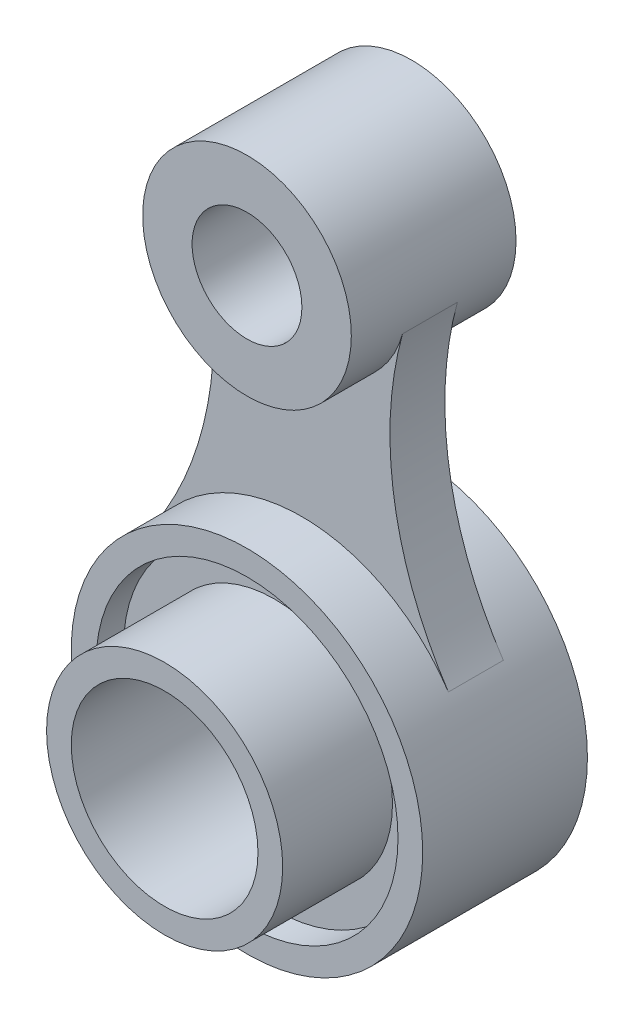
ISO-10303-21;
HEADER;
FILE_DESCRIPTION(('STEP AP214'),'2;1');
FILE_NAME('part.step','',(''),(''),'','','');
FILE_SCHEMA(('AUTOMOTIVE_DESIGN { 1 0 10303 214 1 1 1 1 }'));
ENDSEC;
DATA;
#1=APPLICATION_CONTEXT('core data for automotive mechanical design processes');
#2=APPLICATION_PROTOCOL_DEFINITION('international standard','automotive_design',2000,#1);
#3=PRODUCT_CONTEXT('',#1,'mechanical');
#4=PRODUCT('Part','Part','',(#3));
#5=PRODUCT_RELATED_PRODUCT_CATEGORY('part','',(#4));
#6=PRODUCT_DEFINITION_FORMATION('','',#4);
#7=PRODUCT_DEFINITION_CONTEXT('part definition',#1,'design');
#8=PRODUCT_DEFINITION('design','',#6,#7);
#9=PRODUCT_DEFINITION_SHAPE('','',#8);
#10=(LENGTH_UNIT() NAMED_UNIT(*) SI_UNIT(.MILLI.,.METRE.));
#11=(NAMED_UNIT(*) PLANE_ANGLE_UNIT() SI_UNIT($,.RADIAN.));
#12=(NAMED_UNIT(*) SI_UNIT($,.STERADIAN.) SOLID_ANGLE_UNIT());
#13=UNCERTAINTY_MEASURE_WITH_UNIT(LENGTH_MEASURE(1.E-05),#10,'distance_accuracy_value','');
#14=(GEOMETRIC_REPRESENTATION_CONTEXT(3) GLOBAL_UNCERTAINTY_ASSIGNED_CONTEXT((#13)) GLOBAL_UNIT_ASSIGNED_CONTEXT((#10,
#11,#12)) REPRESENTATION_CONTEXT('',''));
#15=CARTESIAN_POINT('',(0.,0.,0.));
#16=DIRECTION('',(0.,0.,1.));
#17=DIRECTION('',(1.,0.,0.));
#18=AXIS2_PLACEMENT_3D('',#15,#16,#17);
#19=CARTESIAN_POINT('',(0.,0.,10.));
#20=DIRECTION('',(0.,0.,1.));
#21=DIRECTION('',(1.,0.,0.));
#22=AXIS2_PLACEMENT_3D('',#19,#20,#21);
#23=PLANE('',#22);
#24=CARTESIAN_POINT('',(0.,0.,10.));
#25=DIRECTION('',(0.,0.,1.));
#26=DIRECTION('',(1.,0.,0.));
#27=AXIS2_PLACEMENT_3D('',#24,#25,#26);
#28=CIRCLE('',#27,27.5);
#29=CARTESIAN_POINT('',(27.5,0.,10.));
#30=VERTEX_POINT('',#29);
#31=EDGE_CURVE('E12',#30,#30,#28,.T.);
#32=ORIENTED_EDGE('',*,*,#31,.T.);
#33=EDGE_LOOP('',(#32));
#34=FACE_BOUND('',#33,.T.);
#35=CARTESIAN_POINT('',(0.,0.,10.));
#36=DIRECTION('',(0.,0.,1.));
#37=DIRECTION('',(1.,0.,0.));
#38=AXIS2_PLACEMENT_3D('',#35,#36,#37);
#39=CIRCLE('',#38,21.5);
#40=CARTESIAN_POINT('',(21.5,0.,10.));
#41=VERTEX_POINT('',#40);
#42=EDGE_CURVE('E155',#41,#41,#39,.T.);
#43=ORIENTED_EDGE('',*,*,#42,.F.);
#44=EDGE_LOOP('',(#43));
#45=FACE_BOUND('',#44,.T.);
#46=ADVANCED_FACE('F52',(#34,#45),#23,.T.);
#47=CARTESIAN_POINT('',(0.,0.,15.));
#48=DIRECTION('',(0.,0.,-1.));
#49=DIRECTION('',(-1.,0.,0.));
#50=AXIS2_PLACEMENT_3D('',#47,#48,#49);
#51=CYLINDRICAL_SURFACE('',#50,27.5);
#52=ORIENTED_EDGE('',*,*,#31,.F.);
#53=EDGE_LOOP('',(#52));
#54=FACE_BOUND('',#53,.T.);
#55=CARTESIAN_POINT('',(0.,0.,15.));
#56=DIRECTION('',(0.,0.,1.));
#57=DIRECTION('',(1.,0.,0.));
#58=AXIS2_PLACEMENT_3D('',#55,#56,#57);
#59=CIRCLE('',#58,27.5);
#60=CARTESIAN_POINT('',(27.5,0.,15.));
#61=VERTEX_POINT('',#60);
#62=EDGE_CURVE('E127',#61,#61,#59,.T.);
#63=ORIENTED_EDGE('',*,*,#62,.T.);
#64=EDGE_LOOP('',(#63));
#65=FACE_BOUND('',#64,.T.);
#66=ADVANCED_FACE('F54',(#54,#65),#51,.F.);
#67=CARTESIAN_POINT('',(0.,0.,15.));
#68=DIRECTION('',(0.,0.,-1.));
#69=DIRECTION('',(-1.,0.,0.));
#70=AXIS2_PLACEMENT_3D('',#67,#68,#69);
#71=CYLINDRICAL_SURFACE('',#70,32.);
#72=DIRECTION('',(0.,0.,-1.));
#73=VECTOR('',#72,1.);
#74=CARTESIAN_POINT('',(26.6783026465097,17.6711111111111,5.));
#75=LINE('',#74,#73);
#76=CARTESIAN_POINT('',(26.6783026465097,17.6711111111111,5.));
#77=VERTEX_POINT('',#76);
#78=CARTESIAN_POINT('',(26.6783026465097,17.6711111111111,-5.));
#79=VERTEX_POINT('',#78);
#80=EDGE_CURVE('E68',#77,#79,#75,.T.);
#81=ORIENTED_EDGE('',*,*,#80,.F.);
#82=CARTESIAN_POINT('',(0.,0.,5.));
#83=DIRECTION('',(0.,0.,1.));
#84=DIRECTION('',(1.,0.,0.));
#85=AXIS2_PLACEMENT_3D('',#82,#83,#84);
#86=CIRCLE('',#85,32.);
#87=CARTESIAN_POINT('',(-26.6783026465097,17.6711111111111,5.));
#88=VERTEX_POINT('',#87);
#89=EDGE_CURVE('E75',#77,#88,#86,.T.);
#90=ORIENTED_EDGE('',*,*,#89,.T.);
#91=DIRECTION('',(0.,0.,-1.));
#92=VECTOR('',#91,1.);
#93=CARTESIAN_POINT('',(-26.6783026465097,17.6711111111111,5.));
#94=LINE('',#93,#92);
#95=CARTESIAN_POINT('',(-26.6783026465097,17.6711111111111,-5.));
#96=VERTEX_POINT('',#95);
#97=EDGE_CURVE('E114',#88,#96,#94,.T.);
#98=ORIENTED_EDGE('',*,*,#97,.T.);
#99=CARTESIAN_POINT('',(0.,0.,-5.));
#100=DIRECTION('',(0.,0.,1.));
#101=DIRECTION('',(1.,0.,0.));
#102=AXIS2_PLACEMENT_3D('',#99,#100,#101);
#103=CIRCLE('',#102,32.);
#104=EDGE_CURVE('E118',#79,#96,#103,.T.);
#105=ORIENTED_EDGE('',*,*,#104,.F.);
#106=EDGE_LOOP('',(#81,#90,#98,#105));
#107=FACE_BOUND('',#106,.T.);
#108=CARTESIAN_POINT('',(0.,0.,15.));
#109=DIRECTION('',(0.,0.,1.));
#110=DIRECTION('',(1.,0.,0.));
#111=AXIS2_PLACEMENT_3D('',#108,#109,#110);
#112=CIRCLE('',#111,32.);
#113=CARTESIAN_POINT('',(32.,0.,15.));
#114=VERTEX_POINT('',#113);
#115=EDGE_CURVE('E63',#114,#114,#112,.T.);
#116=ORIENTED_EDGE('',*,*,#115,.F.);
#117=EDGE_LOOP('',(#116));
#118=FACE_BOUND('',#117,.T.);
#119=CARTESIAN_POINT('',(0.,0.,-15.));
#120=DIRECTION('',(0.,0.,1.));
#121=DIRECTION('',(1.,0.,0.));
#122=AXIS2_PLACEMENT_3D('',#119,#120,#121);
#123=CIRCLE('',#122,32.);
#124=CARTESIAN_POINT('',(32.,0.,-15.));
#125=VERTEX_POINT('',#124);
#126=EDGE_CURVE('E124',#125,#125,#123,.T.);
#127=ORIENTED_EDGE('',*,*,#126,.T.);
#128=EDGE_LOOP('',(#127));
#129=FACE_BOUND('',#128,.T.);
#130=ADVANCED_FACE('F132',(#107,#118,#129),#71,.T.);
#131=CARTESIAN_POINT('',(0.,0.,15.));
#132=DIRECTION('',(0.,0.,1.));
#133=DIRECTION('',(1.,0.,0.));
#134=AXIS2_PLACEMENT_3D('',#131,#132,#133);
#135=PLANE('',#134);
#136=ORIENTED_EDGE('',*,*,#62,.F.);
#137=EDGE_LOOP('',(#136));
#138=FACE_BOUND('',#137,.T.);
#139=ORIENTED_EDGE('',*,*,#115,.T.);
#140=EDGE_LOOP('',(#139));
#141=FACE_BOUND('',#140,.T.);
#142=ADVANCED_FACE('F137',(#138,#141),#135,.T.);
#143=CARTESIAN_POINT('',(0.,0.,-15.));
#144=DIRECTION('',(0.,0.,1.));
#145=DIRECTION('',(1.,0.,0.));
#146=AXIS2_PLACEMENT_3D('',#143,#144,#145);
#147=PLANE('',#146);
#148=ORIENTED_EDGE('',*,*,#126,.F.);
#149=EDGE_LOOP('',(#148));
#150=FACE_BOUND('',#149,.T.);
#151=CARTESIAN_POINT('',(0.,0.,-15.));
#152=DIRECTION('',(0.,0.,1.));
#153=DIRECTION('',(1.,0.,0.));
#154=AXIS2_PLACEMENT_3D('',#151,#152,#153);
#155=CIRCLE('',#154,17.);
#156=CARTESIAN_POINT('',(17.,0.,-15.));
#157=VERTEX_POINT('',#156);
#158=EDGE_CURVE('E141',#157,#157,#155,.T.);
#159=ORIENTED_EDGE('',*,*,#158,.T.);
#160=EDGE_LOOP('',(#159));
#161=FACE_BOUND('',#160,.T.);
#162=ADVANCED_FACE('F131',(#150,#161),#147,.F.);
#163=CARTESIAN_POINT('',(80.034907939529,53.0133333333333,5.));
#164=DIRECTION('',(0.,0.,-1.));
#165=DIRECTION('',(-1.,0.,0.));
#166=AXIS2_PLACEMENT_3D('',#163,#164,#165);
#167=CYLINDRICAL_SURFACE('',#166,64.);
#168=CARTESIAN_POINT('',(80.034907939529,53.0133333333333,-5.));
#169=DIRECTION('',(0.,0.,1.));
#170=DIRECTION('',(1.,0.,0.));
#171=AXIS2_PLACEMENT_3D('',#168,#169,#170);
#172=CIRCLE('',#171,64.);
#173=CARTESIAN_POINT('',(18.3212439861572,69.9669076305221,-5.));
#174=VERTEX_POINT('',#173);
#175=EDGE_CURVE('E102',#174,#79,#172,.T.);
#176=ORIENTED_EDGE('',*,*,#175,.F.);
#177=DIRECTION('',(0.,0.,-1.));
#178=VECTOR('',#177,1.);
#179=CARTESIAN_POINT('',(18.3212439861572,69.9669076305221,5.));
#180=LINE('',#179,#178);
#181=CARTESIAN_POINT('',(18.3212439861572,69.9669076305221,5.));
#182=VERTEX_POINT('',#181);
#183=EDGE_CURVE('E98',#182,#174,#180,.T.);
#184=ORIENTED_EDGE('',*,*,#183,.F.);
#185=CARTESIAN_POINT('',(80.034907939529,53.0133333333333,5.));
#186=DIRECTION('',(0.,0.,1.));
#187=DIRECTION('',(1.,0.,0.));
#188=AXIS2_PLACEMENT_3D('',#185,#186,#187);
#189=CIRCLE('',#188,64.);
#190=EDGE_CURVE('E117',#182,#77,#189,.T.);
#191=ORIENTED_EDGE('',*,*,#190,.T.);
#192=ORIENTED_EDGE('',*,*,#80,.T.);
#193=EDGE_LOOP('',(#176,#184,#191,#192));
#194=FACE_BOUND('',#193,.T.);
#195=ADVANCED_FACE('F138',(#194),#167,.F.);
#196=CARTESIAN_POINT('',(-80.034907939529,53.0133333333333,5.));
#197=DIRECTION('',(0.,0.,-1.));
#198=DIRECTION('',(-1.,0.,0.));
#199=AXIS2_PLACEMENT_3D('',#196,#197,#198);
#200=CYLINDRICAL_SURFACE('',#199,64.);
#201=CARTESIAN_POINT('',(-80.034907939529,53.0133333333333,-5.));
#202=DIRECTION('',(0.,0.,1.));
#203=DIRECTION('',(1.,0.,0.));
#204=AXIS2_PLACEMENT_3D('',#201,#202,#203);
#205=CIRCLE('',#204,64.);
#206=CARTESIAN_POINT('',(-18.3212439861572,69.9669076305221,-5.));
#207=VERTEX_POINT('',#206);
#208=EDGE_CURVE('E103',#207,#96,#205,.F.);
#209=ORIENTED_EDGE('',*,*,#208,.T.);
#210=ORIENTED_EDGE('',*,*,#97,.F.);
#211=CARTESIAN_POINT('',(-80.034907939529,53.0133333333333,5.));
#212=DIRECTION('',(0.,0.,1.));
#213=DIRECTION('',(1.,0.,0.));
#214=AXIS2_PLACEMENT_3D('',#211,#212,#213);
#215=CIRCLE('',#214,64.);
#216=CARTESIAN_POINT('',(-18.3212439861572,69.9669076305221,5.));
#217=VERTEX_POINT('',#216);
#218=EDGE_CURVE('E112',#217,#88,#215,.F.);
#219=ORIENTED_EDGE('',*,*,#218,.F.);
#220=DIRECTION('',(0.,0.,-1.));
#221=VECTOR('',#220,1.);
#222=CARTESIAN_POINT('',(-18.3212439861572,69.9669076305221,5.));
#223=LINE('',#222,#221);
#224=EDGE_CURVE('E92',#217,#207,#223,.T.);
#225=ORIENTED_EDGE('',*,*,#224,.T.);
#226=EDGE_LOOP('',(#209,#210,#219,#225));
#227=FACE_BOUND('',#226,.T.);
#228=ADVANCED_FACE('F107',(#227),#200,.F.);
#229=CARTESIAN_POINT('',(0.,0.,5.));
#230=DIRECTION('',(0.,0.,1.));
#231=DIRECTION('',(1.,0.,0.));
#232=AXIS2_PLACEMENT_3D('',#229,#230,#231);
#233=PLANE('',#232);
#234=ORIENTED_EDGE('',*,*,#89,.F.);
#235=ORIENTED_EDGE('',*,*,#190,.F.);
#236=CARTESIAN_POINT('',(0.,75.,5.));
#237=DIRECTION('',(0.,0.,1.));
#238=DIRECTION('',(1.,0.,0.));
#239=AXIS2_PLACEMENT_3D('',#236,#237,#238);
#240=CIRCLE('',#239,19.);
#241=EDGE_CURVE('E167',#217,#182,#240,.T.);
#242=ORIENTED_EDGE('',*,*,#241,.F.);
#243=ORIENTED_EDGE('',*,*,#218,.T.);
#244=EDGE_LOOP('',(#234,#235,#242,#243));
#245=FACE_BOUND('',#244,.T.);
#246=ADVANCED_FACE('F174',(#245),#233,.T.);
#247=CARTESIAN_POINT('',(0.,0.,-5.));
#248=DIRECTION('',(0.,0.,1.));
#249=DIRECTION('',(1.,0.,0.));
#250=AXIS2_PLACEMENT_3D('',#247,#248,#249);
#251=PLANE('',#250);
#252=ORIENTED_EDGE('',*,*,#104,.T.);
#253=ORIENTED_EDGE('',*,*,#208,.F.);
#254=CARTESIAN_POINT('',(0.,75.,-5.));
#255=DIRECTION('',(0.,0.,1.));
#256=DIRECTION('',(1.,0.,0.));
#257=AXIS2_PLACEMENT_3D('',#254,#255,#256);
#258=CIRCLE('',#257,19.);
#259=EDGE_CURVE('E93',#207,#174,#258,.T.);
#260=ORIENTED_EDGE('',*,*,#259,.T.);
#261=ORIENTED_EDGE('',*,*,#175,.T.);
#262=EDGE_LOOP('',(#252,#253,#260,#261));
#263=FACE_BOUND('',#262,.T.);
#264=ADVANCED_FACE('F113',(#263),#251,.F.);
#265=CARTESIAN_POINT('',(0.,75.,15.));
#266=DIRECTION('',(0.,0.,-1.));
#267=DIRECTION('',(-1.,0.,0.));
#268=AXIS2_PLACEMENT_3D('',#265,#266,#267);
#269=CYLINDRICAL_SURFACE('',#268,19.);
#270=ORIENTED_EDGE('',*,*,#241,.T.);
#271=ORIENTED_EDGE('',*,*,#183,.T.);
#272=ORIENTED_EDGE('',*,*,#259,.F.);
#273=ORIENTED_EDGE('',*,*,#224,.F.);
#274=EDGE_LOOP('',(#270,#271,#272,#273));
#275=FACE_BOUND('',#274,.T.);
#276=CARTESIAN_POINT('',(0.,75.,15.));
#277=DIRECTION('',(0.,0.,1.));
#278=DIRECTION('',(1.,0.,0.));
#279=AXIS2_PLACEMENT_3D('',#276,#277,#278);
#280=CIRCLE('',#279,19.);
#281=CARTESIAN_POINT('',(19.,75.,15.));
#282=VERTEX_POINT('',#281);
#283=EDGE_CURVE('E156',#282,#282,#280,.T.);
#284=ORIENTED_EDGE('',*,*,#283,.F.);
#285=EDGE_LOOP('',(#284));
#286=FACE_BOUND('',#285,.T.);
#287=CARTESIAN_POINT('',(0.,75.,-15.));
#288=DIRECTION('',(0.,0.,1.));
#289=DIRECTION('',(1.,0.,0.));
#290=AXIS2_PLACEMENT_3D('',#287,#288,#289);
#291=CIRCLE('',#290,19.);
#292=CARTESIAN_POINT('',(19.,75.,-15.));
#293=VERTEX_POINT('',#292);
#294=EDGE_CURVE('E144',#293,#293,#291,.T.);
#295=ORIENTED_EDGE('',*,*,#294,.T.);
#296=EDGE_LOOP('',(#295));
#297=FACE_BOUND('',#296,.T.);
#298=ADVANCED_FACE('F91',(#275,#286,#297),#269,.T.);
#299=CARTESIAN_POINT('',(0.,75.,15.));
#300=DIRECTION('',(0.,0.,-1.));
#301=DIRECTION('',(-1.,0.,0.));
#302=AXIS2_PLACEMENT_3D('',#299,#300,#301);
#303=CYLINDRICAL_SURFACE('',#302,10.);
#304=CARTESIAN_POINT('',(0.,75.,15.));
#305=DIRECTION('',(0.,0.,1.));
#306=DIRECTION('',(1.,0.,0.));
#307=AXIS2_PLACEMENT_3D('',#304,#305,#306);
#308=CIRCLE('',#307,10.);
#309=CARTESIAN_POINT('',(10.,75.,15.));
#310=VERTEX_POINT('',#309);
#311=EDGE_CURVE('E157',#310,#310,#308,.T.);
#312=ORIENTED_EDGE('',*,*,#311,.T.);
#313=EDGE_LOOP('',(#312));
#314=FACE_BOUND('',#313,.T.);
#315=CARTESIAN_POINT('',(0.,75.,-15.));
#316=DIRECTION('',(0.,0.,1.));
#317=DIRECTION('',(1.,0.,0.));
#318=AXIS2_PLACEMENT_3D('',#315,#316,#317);
#319=CIRCLE('',#318,10.);
#320=CARTESIAN_POINT('',(10.,75.,-15.));
#321=VERTEX_POINT('',#320);
#322=EDGE_CURVE('E149',#321,#321,#319,.T.);
#323=ORIENTED_EDGE('',*,*,#322,.F.);
#324=EDGE_LOOP('',(#323));
#325=FACE_BOUND('',#324,.T.);
#326=ADVANCED_FACE('F204',(#314,#325),#303,.F.);
#327=CARTESIAN_POINT('',(0.,0.,15.));
#328=DIRECTION('',(0.,0.,1.));
#329=DIRECTION('',(1.,0.,0.));
#330=AXIS2_PLACEMENT_3D('',#327,#328,#329);
#331=PLANE('',#330);
#332=ORIENTED_EDGE('',*,*,#283,.T.);
#333=EDGE_LOOP('',(#332));
#334=FACE_BOUND('',#333,.T.);
#335=ORIENTED_EDGE('',*,*,#311,.F.);
#336=EDGE_LOOP('',(#335));
#337=FACE_BOUND('',#336,.T.);
#338=ADVANCED_FACE('F203',(#334,#337),#331,.T.);
#339=CARTESIAN_POINT('',(0.,0.,-15.));
#340=DIRECTION('',(0.,0.,1.));
#341=DIRECTION('',(1.,0.,0.));
#342=AXIS2_PLACEMENT_3D('',#339,#340,#341);
#343=PLANE('',#342);
#344=ORIENTED_EDGE('',*,*,#294,.F.);
#345=EDGE_LOOP('',(#344));
#346=FACE_BOUND('',#345,.T.);
#347=ORIENTED_EDGE('',*,*,#322,.T.);
#348=EDGE_LOOP('',(#347));
#349=FACE_BOUND('',#348,.T.);
#350=ADVANCED_FACE('F199',(#346,#349),#343,.F.);
#351=CARTESIAN_POINT('',(0.,0.,-15.));
#352=DIRECTION('',(0.,0.,1.));
#353=DIRECTION('',(1.,0.,0.));
#354=AXIS2_PLACEMENT_3D('',#351,#352,#353);
#355=CYLINDRICAL_SURFACE('',#354,17.);
#356=ORIENTED_EDGE('',*,*,#158,.F.);
#357=EDGE_LOOP('',(#356));
#358=FACE_BOUND('',#357,.T.);
#359=CARTESIAN_POINT('',(0.,0.,30.));
#360=DIRECTION('',(0.,0.,1.));
#361=DIRECTION('',(1.,0.,0.));
#362=AXIS2_PLACEMENT_3D('',#359,#360,#361);
#363=CIRCLE('',#362,17.);
#364=CARTESIAN_POINT('',(17.,0.,30.));
#365=VERTEX_POINT('',#364);
#366=EDGE_CURVE('E432',#365,#365,#363,.T.);
#367=ORIENTED_EDGE('',*,*,#366,.T.);
#368=EDGE_LOOP('',(#367));
#369=FACE_BOUND('',#368,.T.);
#370=ADVANCED_FACE('F198',(#358,#369),#355,.F.);
#371=CARTESIAN_POINT('',(0.,0.,30.));
#372=DIRECTION('',(0.,0.,1.));
#373=DIRECTION('',(1.,0.,0.));
#374=AXIS2_PLACEMENT_3D('',#371,#372,#373);
#375=PLANE('',#374);
#376=CARTESIAN_POINT('',(0.,0.,30.));
#377=DIRECTION('',(0.,0.,1.));
#378=DIRECTION('',(1.,0.,0.));
#379=AXIS2_PLACEMENT_3D('',#376,#377,#378);
#380=CIRCLE('',#379,21.5);
#381=CARTESIAN_POINT('',(21.5,0.,30.));
#382=VERTEX_POINT('',#381);
#383=EDGE_CURVE('E148',#382,#382,#380,.T.);
#384=ORIENTED_EDGE('',*,*,#383,.T.);
#385=EDGE_LOOP('',(#384));
#386=FACE_BOUND('',#385,.T.);
#387=ORIENTED_EDGE('',*,*,#366,.F.);
#388=EDGE_LOOP('',(#387));
#389=FACE_BOUND('',#388,.T.);
#390=ADVANCED_FACE('F200',(#386,#389),#375,.T.);
#391=CARTESIAN_POINT('',(0.,0.,30.));
#392=DIRECTION('',(0.,0.,-1.));
#393=DIRECTION('',(-1.,0.,0.));
#394=AXIS2_PLACEMENT_3D('',#391,#392,#393);
#395=CYLINDRICAL_SURFACE('',#394,21.5);
#396=ORIENTED_EDGE('',*,*,#383,.F.);
#397=EDGE_LOOP('',(#396));
#398=FACE_BOUND('',#397,.T.);
#399=ORIENTED_EDGE('',*,*,#42,.T.);
#400=EDGE_LOOP('',(#399));
#401=FACE_BOUND('',#400,.T.);
#402=ADVANCED_FACE('F192',(#398,#401),#395,.T.);
#403=CLOSED_SHELL('',(#46,#66,#130,#142,#162,#195,#228,#246,#264,#298,#326,#338,#350,#370,#390,#402));
#404=MANIFOLD_SOLID_BREP('B2',#403);
#405=ADVANCED_BREP_SHAPE_REPRESENTATION('',(#18,#404),#14);
#406=SHAPE_DEFINITION_REPRESENTATION(#9,#405);
ENDSEC;
END-ISO-10303-21;
